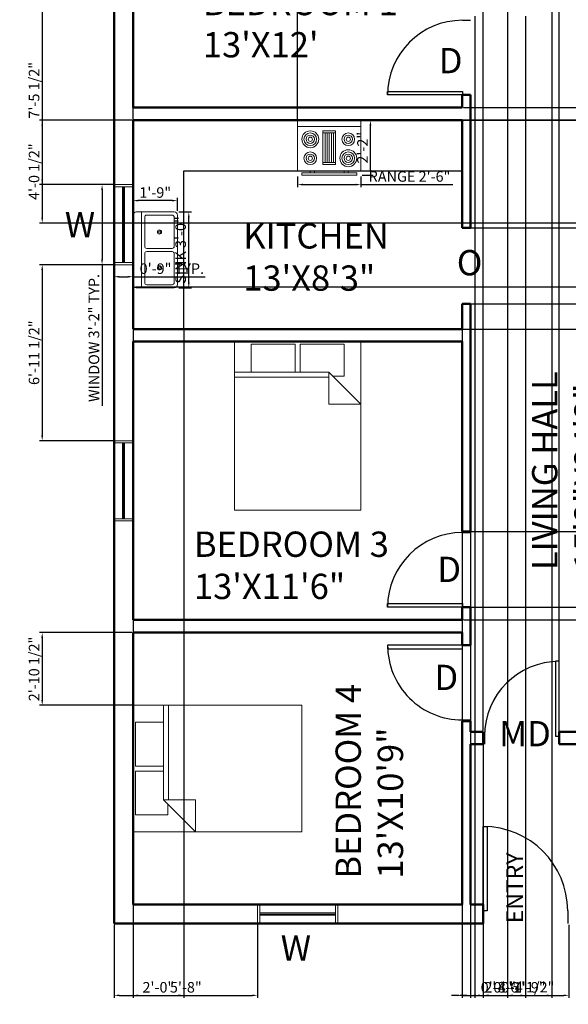
# Model space of a CAD drawing. Units: inches. Extents: x 2050 to 2529, y 1266 to 1968.
# Tile 1 of 5: x 2050 to 2310, y 1266 to 1733. Entities that reach past the tile are written whole.
import ezdxf

# ---------------------------------------------------------------- set-up
doc = ezdxf.new("R2010")
doc.units = ezdxf.units.IN
for name, color, linetype, lineweight in [('A-ANNO-DIMS', 2, 'Continuous', 18), ('A-ANNO-TEXT', 7, 'Continuous', 18), ('A-AREA-IDEN', 7, 'Continuous', 25), ('A-DOOR', 3, 'Continuous', 25), ('A-EQPM', 9, 'Continuous', 18), ('A-FLOR-CABN', 8, 'Continuous', 25), ('A-FLOR-FIXT', 9, 'Continuous', 18), ('A-FURN', 8, 'Continuous', 18), ('A-GLAZ', 4, 'Continuous', 18), ('A-WALL', 7, 'Continuous', 50)]:
    doc.layers.add(name, color=color, linetype=linetype, lineweight=lineweight)
doc.styles.get("Standard").update_dxf_attribs({"font": 'arial.ttf'})
doc.dimstyles.new('ISO-25', dxfattribs={"dimtxt": 5, "dimasz": 2.5, "dimexe": 1.25, "dimexo": 0.625, "dimtad": 1, "dimlunit": 3, "dimtxsty": 'Standard', "dimcen": 2.5, "dimadec": 0, "dimazin": 0, "dimtfac": 1, "dimtmove": 0, "dimatfit": 3, "dimfxl": 1, "dimarcsym": 0})

# ---------------------------------------------------------------- blocks, each defined once
blk = doc.blocks.new('*U4')
for p, q in [((0, 0), (0, -100)), ((-900, 0), (-900, -100))]:
    blk.add_line(p, q)
blk.add_lwpolyline([(0, 0), (0, 900), (-43.75, 900), (-43.75, 0)], close=True)
blk.add_arc((0, 0), 900, 90, 180)
blk = doc.blocks.new('*U5')
for p, q in [((-900, 0), (-900, 100)), ((0, 0), (0, 100))]:
    blk.add_line(p, q)
blk.add_lwpolyline([(0, 0), (0, -900), (-43.75, -900), (-43.75, 0)], close=True)
blk.add_arc((0, 0), 900, 180, 270)
blk = doc.blocks.new('*U6')
for p, q in [((0, 0), (0, 100)), ((900, 0), (900, 100))]:
    blk.add_line(p, q)
blk.add_lwpolyline([(0, 0), (0, -900), (43.75, -900), (43.75, 0)], close=True)
blk.add_arc((0, 0), 900, 270, 0)
blk = doc.blocks.new('*U10')
for p, q in [((0, 0), (0, -6)), ((40, 0), (40, -6))]:
    blk.add_line(p, q)
blk.add_lwpolyline([(0, 0), (0, 40), (1.75, 40), (1.75, 0)], close=True)
blk.add_arc((0, 0), 40, 0, 90)
blk = doc.blocks.new('Sink-double - 36 in top')
for p, q in [((-18, -4), (18, -4)), ((-0.75, -18.5), (-0.75, -6.5)), ((0.75, -6.5), (0.75, -18.5))]:
    blk.add_line(p, q)
for points in [[(-16.5, 0), (16.5, 0)], [(-18, -19.5), (-18, -1.5)], [(18, -1.5), (18, -19.5)], [(-16.5, -18.5), (-16.5, -6.5)], [(-15.5, -5.5), (-1.75, -5.5)], [(1.75, -5.5), (15.5, -5.5)], [(16.5, -6.5), (16.5, -18.5)], [(16.5, -21), (-16.5, -21)], [(-1.75, -19.5), (-15.5, -19.5)], [(15.5, -19.5), (1.75, -19.5)]]:
    blk.add_lwpolyline(points)
for centre, radius in [((-8.5, -12.5), 1), ((-8.5, -12.5), 0.5), ((8.5, -12.5), 1), ((8.5, -12.5), 0.5)]:
    blk.add_circle(centre, radius)
for centre, radius, start, end in [((-16.5, -1.5), 1.5, 90, 180), ((16.5, -1.5), 1.5, 0, 90), ((-15.5, -6.5), 1, 90, 180), ((-1.75, -6.5), 1, 0, 90), ((1.75, -6.5), 1, 90, 180), ((15.5, -6.5), 1, 0, 90), ((-15.5, -18.5), 1, 180, 270), ((-1.75, -18.5), 1, 270, 0), ((1.75, -18.5), 1, 180, 270), ((15.5, -18.5), 1, 270, 0), ((-16.5, -19.5), 1.5, 180, 270), ((16.5, -19.5), 1.5, 270, 0)]:
    blk.add_arc(centre, radius, start, end)
blk = doc.blocks.new('Range-Oven - 30 in top')
for p, q in [((0, -3), (30, -3)), ((12, -6), (18, -6)), ((13, -20), (13, -6)), ((14, -6), (14, -20)), ((15, -20), (15, -6)), ((16, -6), (16, -20)), ((17, -20), (17, -6)), ((18, -20), (12, -20)), ((6, -24), (6, -25)), ((8, -25), (8, -24)), ((22, -25), (22, -24)), ((24, -24), (24, -25))]:
    blk.add_line(p, q)
for points in [[(0, -24), (0, 0), (30, 0), (30, -24)], [(12, -21), (12, -5), (18, -5), (18, -21)], [(2, -26), (2, -25), (28, -25), (28, -26)]]:
    blk.add_lwpolyline(points, close=True)
for centre, radius in [((6, -9), 4), ((6, -9), 3), ((6, -9), 2), ((6, -9), 1), ((24, -9), 3), ((24, -9), 2), ((24, -9), 1), ((24, -18), 4), ((6, -18), 3), ((6, -18), 2), ((6, -18), 1), ((24, -18), 3), ((24, -18), 2), ((24, -18), 1)]:
    blk.add_circle(centre, radius)
blk = doc.blocks.new('Bed - Queen')
for p, q in [((0, -80.00003), (0, 0)), ((0, 0), (59.99999, 0)), ((59.99999, 0), (59.99999, -80.00003)), ((7.99999, -1.2), (28.79998, -1.2)), ((7.99999, -14.4), (7.99999, -1.2)), ((28.79998, -1.2), (28.79998, -14.4)), ((31.19999, -1.2), (51.99999, -1.2)), ((31.19999, -14.4), (31.19999, -1.2)), ((51.99999, -1.2), (51.99999, -16.4)), ((0, -14.4), (44.8, -14.4)), ((44.8, -16.8), (0, -16.8)), ((59.99999, -29.6), (44.8, -14.4)), ((44.8, -14.4), (44.8, -29.6)), ((51.99999, -16.4), (46.79936, -16.4)), ((44.8, -29.6), (59.99999, -29.6)), ((59.99999, -80.00003), (0, -80.00003))]:
    blk.add_line(p, q)
blk = doc.blocks.new('WIN-36IN')
for p, q in [((0, 9), (0, 0)), ((1, 9), (1, 0)), ((1, 5), (37, 5)), ((37, 9), (37, 0)), ((38, 9), (38, 0)), ((1, 4.5), (37, 4.5)), ((1, 4), (37, 4))]:
    blk.add_line(p, q)
blk = doc.blocks.new('*D26')
at = {"layer": 'A-ANNO-DIMS', "color": 0, "lineweight": -2, "transparency": 16777216}
for p, q in [((2093.67, 1655.22), (2087.34, 1655.22)), ((2088.59, 1652.72), (2088.59, 1619.72)), ((2093.67, 1617.22), (2087.34, 1617.22)), ((2088.59, 1617.22), (2088.59, 1550.2))]:
    blk.add_line(p, q, dxfattribs=at)
at = {"layer": 'A-ANNO-DIMS', "color": 0, "transparency": 16777216}
for points in [[(2088.18, 1652.72), (2089.01, 1652.72), (2088.59, 1655.22)], [(2088.18, 1619.72), (2089.01, 1619.72), (2088.59, 1617.22)]]:
    blk.add_solid(points, dxfattribs=at)
at = {"layer": 'Defpoints', "color": 0, "transparency": 16777216}
for p in [(2094.29, 1655.22), (2088.59, 1617.22), (2094.29, 1617.22)]:
    blk.add_point(p, dxfattribs=at)
at = {"layer": 'A-ANNO-DIMS', "color": 0, "transparency": 16777216, "insert": (2085.38, 1582.46), "char_height": 5, "attachment_point": 5, "rotation": 90}
blk.add_mtext('WINDOW 3\'-2" TYP.', dxfattribs=at)
blk = doc.blocks.new('*D27')
at = {"layer": 'A-ANNO-DIMS', "color": 0, "lineweight": -2, "transparency": 16777216}
for p, q in [((2094.29, 1616.6), (2094.29, 1610.27)), ((2103.29, 1616.6), (2103.29, 1610.27)), ((2096.79, 1611.52), (2100.79, 1611.52)), ((2103.29, 1611.52), (2137.52, 1611.52))]:
    blk.add_line(p, q, dxfattribs=at)
at = {"layer": 'A-ANNO-DIMS', "color": 0, "transparency": 16777216}
for points in [[(2096.79, 1611.94), (2096.79, 1611.1), (2094.29, 1611.52)], [(2100.79, 1611.94), (2100.79, 1611.1), (2103.29, 1611.52)]]:
    blk.add_solid(points, dxfattribs=at)
at = {"layer": 'Defpoints', "color": 0, "transparency": 16777216}
for p in [(2094.29, 1617.22), (2103.29, 1617.22), (2103.29, 1611.52)]:
    blk.add_point(p, dxfattribs=at)
at = {"layer": 'A-ANNO-DIMS', "color": 0, "transparency": 16777216, "insert": (2121.66, 1614.7), "char_height": 5, "attachment_point": 5}
blk.add_mtext('0\'-9" TYP.', dxfattribs=at)
blk = doc.blocks.new('*D34')
at = {"layer": 'A-ANNO-DIMS', "color": 0, "lineweight": -2, "transparency": 16777216}
for p, q in [((2124.92, 1642.22), (2130.94, 1642.22)), ((2129.69, 1608.72), (2129.69, 1639.72)), ((2124.92, 1606.22), (2130.94, 1606.22))]:
    blk.add_line(p, q, dxfattribs=at)
at = {"layer": 'A-ANNO-DIMS', "color": 0, "transparency": 16777216}
for points in [[(2129.28, 1639.72), (2130.11, 1639.72), (2129.69, 1642.22)], [(2129.28, 1608.72), (2130.11, 1608.72), (2129.69, 1606.22)]]:
    blk.add_solid(points, dxfattribs=at)
at = {"layer": 'Defpoints', "color": 0, "transparency": 16777216}
for p in [(2124.29, 1642.22), (2129.69, 1642.22), (2124.29, 1606.22)]:
    blk.add_point(p, dxfattribs=at)
at = {"layer": 'A-ANNO-DIMS', "color": 0, "transparency": 16777216, "insert": (2126.48, 1624.22), "char_height": 5, "attachment_point": 5, "rotation": 90}
blk.add_mtext('SINK 3\'-0"', dxfattribs=at)
blk = doc.blocks.new('*D35')
at = {"layer": 'A-ANNO-DIMS', "color": 0, "lineweight": -2, "transparency": 16777216}
for p, q in [((2103.29, 1642.85), (2103.29, 1648.87)), ((2124.29, 1642.85), (2124.29, 1648.87)), ((2121.79, 1647.62), (2105.79, 1647.62))]:
    blk.add_line(p, q, dxfattribs=at)
at = {"layer": 'A-ANNO-DIMS', "color": 0, "transparency": 16777216}
for points in [[(2105.79, 1648.04), (2105.79, 1647.2), (2103.29, 1647.62)], [(2121.79, 1648.04), (2121.79, 1647.2), (2124.29, 1647.62)]]:
    blk.add_solid(points, dxfattribs=at)
at = {"layer": 'Defpoints', "color": 0, "transparency": 16777216}
for p in [(2103.29, 1647.62), (2103.29, 1642.22), (2124.29, 1642.22)]:
    blk.add_point(p, dxfattribs=at)
at = {"layer": 'A-ANNO-DIMS', "color": 0, "transparency": 16777216, "insert": (2113.79, 1650.8), "char_height": 5, "attachment_point": 5}
blk.add_mtext('1\'-9"', dxfattribs=at)
blk = doc.blocks.new('*D36')
at = {"layer": 'A-ANNO-DIMS', "color": 0, "lineweight": -2, "transparency": 16777216}
for p, q in [((2181.29, 1659.1), (2181.29, 1653.97)), ((2211.29, 1659.1), (2211.29, 1653.97)), ((2183.79, 1655.22), (2208.79, 1655.22)), ((2211.29, 1655.22), (2254.86, 1655.22))]:
    blk.add_line(p, q, dxfattribs=at)
at = {"layer": 'A-ANNO-DIMS', "color": 0, "transparency": 16777216}
for points in [[(2183.79, 1655.64), (2183.79, 1654.8), (2181.29, 1655.22)], [(2208.79, 1655.64), (2208.79, 1654.8), (2211.29, 1655.22)]]:
    blk.add_solid(points, dxfattribs=at)
at = {"layer": 'Defpoints', "color": 0, "transparency": 16777216}
for p in [(2181.29, 1659.72), (2211.29, 1659.72), (2211.29, 1655.22)]:
    blk.add_point(p, dxfattribs=at)
at = {"layer": 'A-ANNO-DIMS', "color": 0, "transparency": 16777216, "insert": (2234.33, 1658.43), "char_height": 5, "attachment_point": 5}
blk.add_mtext('RANGE 2\'-6"', dxfattribs=at)
blk = doc.blocks.new('*D37')
at = {"layer": 'A-ANNO-DIMS', "color": 0, "lineweight": -2, "transparency": 16777216}
for p, q in [((2211.92, 1685.72), (2217.04, 1685.72)), ((2215.79, 1662.22), (2215.79, 1683.22)), ((2211.92, 1659.72), (2217.04, 1659.72))]:
    blk.add_line(p, q, dxfattribs=at)
at = {"layer": 'A-ANNO-DIMS', "color": 0, "transparency": 16777216}
for points in [[(2215.38, 1683.22), (2216.21, 1683.22), (2215.79, 1685.72)], [(2215.38, 1662.22), (2216.21, 1662.22), (2215.79, 1659.72)]]:
    blk.add_solid(points, dxfattribs=at)
at = {"layer": 'Defpoints', "color": 0, "transparency": 16777216}
for p in [(2211.29, 1685.72), (2215.79, 1685.72), (2211.29, 1659.72)]:
    blk.add_point(p, dxfattribs=at)
at = {"layer": 'A-ANNO-DIMS', "color": 0, "transparency": 16777216, "insert": (2212.66, 1672.72), "char_height": 5, "attachment_point": 5, "rotation": 90}
blk.add_mtext('2\'-2"', dxfattribs=at)
blk = doc.blocks.new('*D42')
at = {"layer": 'A-ANNO-DIMS', "color": 0, "lineweight": -2, "transparency": 16777216}
for p, q in [((2103.29, 1586.1), (2103.29, 1269.4)), ((2127.29, 1586.1), (2127.29, 1269.4)), ((2105.79, 1270.65), (2124.79, 1270.65))]:
    blk.add_line(p, q, dxfattribs=at)
at = {"layer": 'A-ANNO-DIMS', "color": 0, "transparency": 16777216}
for points in [[(2105.79, 1271.06), (2105.79, 1270.23), (2103.29, 1270.65)], [(2124.79, 1271.06), (2124.79, 1270.23), (2127.29, 1270.65)]]:
    blk.add_solid(points, dxfattribs=at)
at = {"layer": 'Defpoints', "color": 0, "transparency": 16777216}
for p in [(2103.29, 1586.72), (2127.29, 1586.72), (2127.29, 1270.65)]:
    blk.add_point(p, dxfattribs=at)
at = {"layer": 'A-ANNO-DIMS', "color": 0, "transparency": 16777216, "insert": (2115.29, 1273.82), "char_height": 5, "attachment_point": 5}
blk.add_mtext('2\'-0"', dxfattribs=at)
blk = doc.blocks.new('*D43')
at = {"layer": 'A-ANNO-DIMS', "color": 0, "lineweight": -2, "transparency": 16777216}
for p, q in [((2103.29, 1686.35), (2103.29, 1907.05)), ((2105.79, 1905.8), (2178.79, 1905.8)), ((2181.29, 1686.35), (2181.29, 1907.05))]:
    blk.add_line(p, q, dxfattribs=at)
at = {"layer": 'A-ANNO-DIMS', "color": 0, "transparency": 16777216}
for points in [[(2105.79, 1906.21), (2105.79, 1905.38), (2103.29, 1905.8)], [(2178.79, 1906.21), (2178.79, 1905.38), (2181.29, 1905.8)]]:
    blk.add_solid(points, dxfattribs=at)
at = {"layer": 'Defpoints', "color": 0, "transparency": 16777216}
for p in [(2181.29, 1905.8), (2103.29, 1685.72), (2181.29, 1685.72)]:
    blk.add_point(p, dxfattribs=at)
at = {"layer": 'A-ANNO-DIMS', "color": 0, "transparency": 16777216, "insert": (2142.29, 1908.97), "char_height": 5, "attachment_point": 5}
blk.add_mtext('6\'-6"', dxfattribs=at)
blk = doc.blocks.new('*D44')
at = {"layer": 'A-ANNO-DIMS', "color": 0, "lineweight": -2, "transparency": 16777216}
for p, q in [((2104.36, 1606.66), (2489.62, 1606.66)), ((2488.37, 1589.22), (2488.37, 1604.16)), ((2103.92, 1586.72), (2489.62, 1586.72))]:
    blk.add_line(p, q, dxfattribs=at)
at = {"layer": 'A-ANNO-DIMS', "color": 0, "transparency": 16777216}
for points in [[(2487.95, 1604.16), (2488.79, 1604.16), (2488.37, 1606.66)], [(2487.95, 1589.22), (2488.79, 1589.22), (2488.37, 1586.72)]]:
    blk.add_solid(points, dxfattribs=at)
at = {"layer": 'Defpoints', "color": 0, "transparency": 16777216}
for p in [(2103.73, 1606.66), (2488.37, 1606.66), (2103.29, 1586.72)]:
    blk.add_point(p, dxfattribs=at)
at = {"layer": 'A-ANNO-DIMS', "color": 0, "transparency": 16777216, "insert": (2485.19, 1596.69), "char_height": 5, "attachment_point": 5, "rotation": 90}
blk.add_mtext('1\'-8"', dxfattribs=at)
blk = doc.blocks.new('*D45')
at = {"layer": 'A-ANNO-DIMS', "color": 0, "lineweight": -2, "transparency": 16777216}
for p, q in [((2259.92, 1634.72), (2489.62, 1634.72)), ((2488.37, 1601.22), (2488.37, 1632.22)), ((2259.92, 1598.72), (2489.62, 1598.72))]:
    blk.add_line(p, q, dxfattribs=at)
at = {"layer": 'A-ANNO-DIMS', "color": 0, "transparency": 16777216}
for points in [[(2487.95, 1632.22), (2488.79, 1632.22), (2488.37, 1634.72)], [(2487.95, 1601.22), (2488.79, 1601.22), (2488.37, 1598.72)]]:
    blk.add_solid(points, dxfattribs=at)
at = {"layer": 'Defpoints', "color": 0, "transparency": 16777216}
for p in [(2259.29, 1634.72), (2488.37, 1634.72), (2259.29, 1598.72)]:
    blk.add_point(p, dxfattribs=at)
at = {"layer": 'A-ANNO-DIMS', "color": 0, "transparency": 16777216, "insert": (2485.19, 1616.72), "char_height": 5, "attachment_point": 5, "rotation": 90}
blk.add_mtext('3\'-0"', dxfattribs=at)
blk = doc.blocks.new('*D46')
at = {"layer": 'A-ANNO-DIMS', "color": 0, "lineweight": -2, "transparency": 16777216}
for p, q in [((2259.29, 1598.1), (2259.29, 1269.4)), ((2263.29, 1598.1), (2263.29, 1269.4)), ((2256.79, 1270.65), (2254.29, 1270.65)), ((2259.29, 1270.65), (2263.29, 1270.65)), ((2265.79, 1270.65), (2282.84, 1270.65))]:
    blk.add_line(p, q, dxfattribs=at)
at = {"layer": 'A-ANNO-DIMS', "color": 0, "transparency": 16777216}
for points in [[(2256.79, 1271.06), (2256.79, 1270.23), (2259.29, 1270.65)], [(2265.79, 1271.06), (2265.79, 1270.23), (2263.29, 1270.65)]]:
    blk.add_solid(points, dxfattribs=at)
at = {"layer": 'Defpoints', "color": 0, "transparency": 16777216}
for p in [(2259.29, 1598.72), (2263.29, 1598.72), (2263.29, 1270.65)]:
    blk.add_point(p, dxfattribs=at)
at = {"layer": 'A-ANNO-DIMS', "color": 0, "transparency": 16777216, "insert": (2275.57, 1273.82), "char_height": 5, "attachment_point": 5}
blk.add_mtext('0\'-4"', dxfattribs=at)
blk = doc.blocks.new('*D47')
at = {"layer": 'A-ANNO-DIMS', "color": 0, "lineweight": -2, "transparency": 16777216}
for p, q in [((2488.37, 1598.72), (2488.37, 1615.29)), ((2259.92, 1598.72), (2489.62, 1598.72)), ((2488.37, 1589.22), (2488.37, 1596.22)), ((2259.92, 1586.72), (2489.62, 1586.72))]:
    blk.add_line(p, q, dxfattribs=at)
at = {"layer": 'A-ANNO-DIMS', "color": 0, "transparency": 16777216}
for points in [[(2487.95, 1596.22), (2488.79, 1596.22), (2488.37, 1598.72)], [(2487.95, 1589.22), (2488.79, 1589.22), (2488.37, 1586.72)]]:
    blk.add_solid(points, dxfattribs=at)
at = {"layer": 'Defpoints', "color": 0, "transparency": 16777216}
for p in [(2259.29, 1598.72), (2488.37, 1598.72), (2259.29, 1586.72)]:
    blk.add_point(p, dxfattribs=at)
at = {"layer": 'A-ANNO-DIMS', "color": 0, "transparency": 16777216, "insert": (2485.19, 1608.26), "char_height": 5, "attachment_point": 5, "rotation": 90}
blk.add_mtext('1\'-0"', dxfattribs=at)
blk = doc.blocks.new('*D48')
at = {"layer": 'A-ANNO-DIMS', "color": 0, "lineweight": -2, "transparency": 16777216}
for p, q in [((2488.37, 1694.22), (2488.37, 1711.26)), ((2259.92, 1691.72), (2489.62, 1691.72)), ((2488.37, 1685.72), (2488.37, 1691.72)), ((2259.92, 1685.72), (2489.62, 1685.72)), ((2488.37, 1683.22), (2488.37, 1680.72))]:
    blk.add_line(p, q, dxfattribs=at)
at = {"layer": 'A-ANNO-DIMS', "color": 0, "transparency": 16777216}
for points in [[(2487.95, 1694.22), (2488.79, 1694.22), (2488.37, 1691.72)], [(2487.95, 1683.22), (2488.79, 1683.22), (2488.37, 1685.72)]]:
    blk.add_solid(points, dxfattribs=at)
at = {"layer": 'Defpoints', "color": 0, "transparency": 16777216}
for p in [(2259.29, 1691.72), (2488.37, 1691.72), (2259.29, 1685.72)]:
    blk.add_point(p, dxfattribs=at)
at = {"layer": 'A-ANNO-DIMS', "color": 0, "transparency": 16777216, "insert": (2485.19, 1703.99), "char_height": 5, "attachment_point": 5, "rotation": 90}
blk.add_mtext('0\'-6"', dxfattribs=at)
blk = doc.blocks.new('*D49')
at = {"layer": 'A-ANNO-DIMS', "color": 0, "lineweight": -2, "transparency": 16777216}
for p, q in [((2269.29, 1304.1), (2269.29, 1269.4)), ((2309.85, 1304.1), (2309.85, 1269.4)), ((2271.79, 1270.65), (2307.35, 1270.65))]:
    blk.add_line(p, q, dxfattribs=at)
at = {"layer": 'A-ANNO-DIMS', "color": 0, "transparency": 16777216}
for points in [[(2271.79, 1271.06), (2271.79, 1270.23), (2269.29, 1270.65)], [(2307.35, 1271.06), (2307.35, 1270.23), (2309.85, 1270.65)]]:
    blk.add_solid(points, dxfattribs=at)
at = {"layer": 'Defpoints', "color": 0, "transparency": 16777216}
for p in [(2269.29, 1304.72), (2309.85, 1304.72), (2309.85, 1270.65)]:
    blk.add_point(p, dxfattribs=at)
at = {"layer": 'A-ANNO-DIMS', "color": 0, "transparency": 16777216, "insert": (2289.57, 1273.86), "char_height": 5, "attachment_point": 5}
blk.add_mtext('3\'-4 1/2"', dxfattribs=at)
blk = doc.blocks.new('*D50')
at = {"layer": 'A-ANNO-DIMS', "color": 0, "lineweight": -2, "transparency": 16777216}
for p, q in [((2263.29, 1313.1), (2263.29, 1269.4)), ((2269.29, 1313.1), (2269.29, 1269.4)), ((2260.79, 1270.65), (2258.29, 1270.65)), ((2263.29, 1270.65), (2269.29, 1270.65)), ((2271.79, 1270.65), (2288.84, 1270.65))]:
    blk.add_line(p, q, dxfattribs=at)
at = {"layer": 'A-ANNO-DIMS', "color": 0, "transparency": 16777216}
for points in [[(2260.79, 1271.06), (2260.79, 1270.23), (2263.29, 1270.65)], [(2271.79, 1271.06), (2271.79, 1270.23), (2269.29, 1270.65)]]:
    blk.add_solid(points, dxfattribs=at)
at = {"layer": 'Defpoints', "color": 0, "transparency": 16777216}
for p in [(2263.29, 1313.72), (2269.29, 1313.72), (2269.29, 1270.65)]:
    blk.add_point(p, dxfattribs=at)
at = {"layer": 'A-ANNO-DIMS', "color": 0, "transparency": 16777216, "insert": (2281.57, 1273.82), "char_height": 5, "attachment_point": 5}
blk.add_mtext('0\'-6"', dxfattribs=at)
blk = doc.blocks.new('*D54')
at = {"layer": 'A-ANNO-DIMS', "color": 0, "lineweight": -2, "transparency": 16777216}
for p, q in [((2269.29, 1396.35), (2269.29, 1907.05)), ((2271.79, 1905.8), (2302.79, 1905.8)), ((2305.29, 1396.35), (2305.29, 1907.05))]:
    blk.add_line(p, q, dxfattribs=at)
at = {"layer": 'A-ANNO-DIMS', "color": 0, "transparency": 16777216}
for points in [[(2271.79, 1906.21), (2271.79, 1905.38), (2269.29, 1905.8)], [(2302.79, 1906.21), (2302.79, 1905.38), (2305.29, 1905.8)]]:
    blk.add_solid(points, dxfattribs=at)
at = {"layer": 'Defpoints', "color": 0, "transparency": 16777216}
for p in [(2305.29, 1905.8), (2269.29, 1395.72), (2305.29, 1395.72)]:
    blk.add_point(p, dxfattribs=at)
at = {"layer": 'A-ANNO-DIMS', "color": 0, "transparency": 16777216, "insert": (2287.29, 1908.98), "char_height": 5, "attachment_point": 5}
blk.add_mtext('3\'-0"', dxfattribs=at)
blk = doc.blocks.new('*D55')
at = {"layer": 'A-ANNO-DIMS', "color": 0, "lineweight": -2, "transparency": 16777216}
for p, q in [((2263.29, 1395.1), (2263.29, 1269.4)), ((2269.29, 1395.1), (2269.29, 1269.4)), ((2260.79, 1270.65), (2258.29, 1270.65)), ((2263.29, 1270.65), (2269.29, 1270.65)), ((2271.79, 1270.65), (2288.84, 1270.65))]:
    blk.add_line(p, q, dxfattribs=at)
at = {"layer": 'A-ANNO-DIMS', "color": 0, "transparency": 16777216}
for points in [[(2260.79, 1271.06), (2260.79, 1270.23), (2263.29, 1270.65)], [(2271.79, 1271.06), (2271.79, 1270.23), (2269.29, 1270.65)]]:
    blk.add_solid(points, dxfattribs=at)
at = {"layer": 'Defpoints', "color": 0, "transparency": 16777216}
for p in [(2263.29, 1395.72), (2269.29, 1395.72), (2269.29, 1270.65)]:
    blk.add_point(p, dxfattribs=at)
at = {"layer": 'A-ANNO-DIMS', "color": 0, "transparency": 16777216, "insert": (2281.57, 1273.82), "char_height": 5, "attachment_point": 5}
blk.add_mtext('0\'-6"', dxfattribs=at)
blk = doc.blocks.new('*D58')
at = {"layer": 'A-ANNO-DIMS', "color": 0, "lineweight": -2, "transparency": 16777216}
for p, q in [((2488.37, 1457.22), (2488.37, 1474.26)), ((2259.92, 1454.72), (2489.62, 1454.72)), ((2488.37, 1448.72), (2488.37, 1454.72)), ((2259.92, 1448.72), (2489.62, 1448.72)), ((2488.37, 1446.22), (2488.37, 1443.72))]:
    blk.add_line(p, q, dxfattribs=at)
at = {"layer": 'A-ANNO-DIMS', "color": 0, "transparency": 16777216}
for points in [[(2487.95, 1457.22), (2488.79, 1457.22), (2488.37, 1454.72)], [(2487.95, 1446.22), (2488.79, 1446.22), (2488.37, 1448.72)]]:
    blk.add_solid(points, dxfattribs=at)
at = {"layer": 'Defpoints', "color": 0, "transparency": 16777216}
for p in [(2259.29, 1454.72), (2488.37, 1454.72), (2259.29, 1448.72)]:
    blk.add_point(p, dxfattribs=at)
at = {"layer": 'A-ANNO-DIMS', "color": 0, "transparency": 16777216, "insert": (2485.19, 1466.99), "char_height": 5, "attachment_point": 5, "rotation": 90}
blk.add_mtext('0\'-6"', dxfattribs=at)
blk = doc.blocks.new('*D59')
at = {"layer": 'A-ANNO-DIMS', "color": 0, "lineweight": -2, "transparency": 16777216}
for p, q in [((2259.92, 1490.72), (2489.62, 1490.72)), ((2488.37, 1457.22), (2488.37, 1488.22)), ((2259.92, 1454.72), (2489.62, 1454.72))]:
    blk.add_line(p, q, dxfattribs=at)
at = {"layer": 'A-ANNO-DIMS', "color": 0, "transparency": 16777216}
for points in [[(2487.95, 1488.22), (2488.79, 1488.22), (2488.37, 1490.72)], [(2487.95, 1457.22), (2488.79, 1457.22), (2488.37, 1454.72)]]:
    blk.add_solid(points, dxfattribs=at)
at = {"layer": 'Defpoints', "color": 0, "transparency": 16777216}
for p in [(2259.29, 1490.72), (2488.37, 1490.72), (2259.29, 1454.72)]:
    blk.add_point(p, dxfattribs=at)
at = {"layer": 'A-ANNO-DIMS', "color": 0, "transparency": 16777216, "insert": (2485.19, 1472.72), "char_height": 5, "attachment_point": 5, "rotation": 90}
blk.add_mtext('3\'-0"', dxfattribs=at)
blk = doc.blocks.new('*D60')
at = {"layer": 'A-ANNO-DIMS', "color": 0, "lineweight": -2, "transparency": 16777216}
for p, q in [((2265.29, 1735.1), (2265.29, 1269.4)), ((2289.29, 1735.1), (2289.29, 1269.4)), ((2267.79, 1270.65), (2286.79, 1270.65))]:
    blk.add_line(p, q, dxfattribs=at)
at = {"layer": 'A-ANNO-DIMS', "color": 0, "transparency": 16777216}
for points in [[(2267.79, 1271.06), (2267.79, 1270.23), (2265.29, 1270.65)], [(2286.79, 1271.06), (2286.79, 1270.23), (2289.29, 1270.65)]]:
    blk.add_solid(points, dxfattribs=at)
at = {"layer": 'Defpoints', "color": 0, "transparency": 16777216}
for p in [(2265.29, 1735.72), (2289.29, 1735.72), (2289.29, 1270.65)]:
    blk.add_point(p, dxfattribs=at)
at = {"layer": 'A-ANNO-DIMS', "color": 0, "transparency": 16777216, "insert": (2277.29, 1273.82), "char_height": 5, "attachment_point": 5}
blk.add_mtext('2\'-0"', dxfattribs=at)
blk = doc.blocks.new('*D64')
at = {"layer": 'A-ANNO-DIMS', "color": 0, "lineweight": -2, "transparency": 16777216}
for p, q in [((2280.79, 1835.1), (2280.79, 1269.4)), ((2301.79, 1835.1), (2301.79, 1269.4)), ((2283.29, 1270.65), (2299.29, 1270.65))]:
    blk.add_line(p, q, dxfattribs=at)
at = {"layer": 'A-ANNO-DIMS', "color": 0, "transparency": 16777216}
for points in [[(2283.29, 1271.06), (2283.29, 1270.23), (2280.79, 1270.65)], [(2299.29, 1271.06), (2299.29, 1270.23), (2301.79, 1270.65)]]:
    blk.add_solid(points, dxfattribs=at)
at = {"layer": 'Defpoints', "color": 0, "transparency": 16777216}
for p in [(2280.79, 1835.72), (2301.79, 1835.72), (2301.79, 1270.65)]:
    blk.add_point(p, dxfattribs=at)
at = {"layer": 'A-ANNO-DIMS', "color": 0, "transparency": 16777216, "insert": (2291.29, 1273.82), "char_height": 5, "attachment_point": 5}
blk.add_mtext('1\'-9"', dxfattribs=at)
blk = doc.blocks.new('*D67')
at = {"layer": 'A-ANNO-DIMS', "color": 0, "lineweight": -2, "transparency": 16777216}
for p, q in [((2093.67, 1744.72), (2058.97, 1744.72)), ((2060.22, 1742.22), (2060.22, 1657.72)), ((2093.67, 1655.22), (2058.97, 1655.22))]:
    blk.add_line(p, q, dxfattribs=at)
at = {"layer": 'A-ANNO-DIMS', "color": 0, "transparency": 16777216}
for points in [[(2059.8, 1742.22), (2060.64, 1742.22), (2060.22, 1744.72)], [(2059.8, 1657.72), (2060.64, 1657.72), (2060.22, 1655.22)]]:
    blk.add_solid(points, dxfattribs=at)
at = {"layer": 'Defpoints', "color": 0, "transparency": 16777216}
for p in [(2094.29, 1744.72), (2060.22, 1655.22), (2094.29, 1655.22)]:
    blk.add_point(p, dxfattribs=at)
at = {"layer": 'A-ANNO-DIMS', "color": 0, "transparency": 16777216, "insert": (2057.01, 1699.97), "char_height": 5, "attachment_point": 5, "rotation": 90}
blk.add_mtext('7\'-5 1/2"', dxfattribs=at)
blk = doc.blocks.new('*D68')
at = {"layer": 'A-ANNO-DIMS', "color": 0, "lineweight": -2, "transparency": 16777216}
for p, q in [((2093.67, 1617.22), (2058.97, 1617.22)), ((2060.22, 1614.72), (2060.22, 1536.22)), ((2093.67, 1533.72), (2058.97, 1533.72))]:
    blk.add_line(p, q, dxfattribs=at)
at = {"layer": 'A-ANNO-DIMS', "color": 0, "transparency": 16777216}
for points in [[(2059.8, 1614.72), (2060.64, 1614.72), (2060.22, 1617.22)], [(2059.8, 1536.22), (2060.64, 1536.22), (2060.22, 1533.72)]]:
    blk.add_solid(points, dxfattribs=at)
at = {"layer": 'Defpoints', "color": 0, "transparency": 16777216}
for p in [(2094.29, 1617.22), (2060.22, 1533.72), (2094.29, 1533.72)]:
    blk.add_point(p, dxfattribs=at)
at = {"layer": 'A-ANNO-DIMS', "color": 0, "transparency": 16777216, "insert": (2057.01, 1575.47), "char_height": 5, "attachment_point": 5, "rotation": 90}
blk.add_mtext('6\'-11 1/2"', dxfattribs=at)
blk = doc.blocks.new('*D69')
at = {"layer": 'A-ANNO-DIMS', "color": 0, "lineweight": -2, "transparency": 16777216}
for p, q in [((2094.29, 1304.1), (2094.29, 1269.4)), ((2162.29, 1304.1), (2162.29, 1269.4)), ((2096.79, 1270.65), (2159.79, 1270.65))]:
    blk.add_line(p, q, dxfattribs=at)
at = {"layer": 'A-ANNO-DIMS', "color": 0, "transparency": 16777216}
for points in [[(2096.79, 1271.06), (2096.79, 1270.23), (2094.29, 1270.65)], [(2159.79, 1271.06), (2159.79, 1270.23), (2162.29, 1270.65)]]:
    blk.add_solid(points, dxfattribs=at)
at = {"layer": 'Defpoints', "color": 0, "transparency": 16777216}
for p in [(2094.29, 1304.72), (2162.29, 1304.72), (2162.29, 1270.65)]:
    blk.add_point(p, dxfattribs=at)
at = {"layer": 'A-ANNO-DIMS', "color": 0, "transparency": 16777216, "insert": (2128.29, 1273.82), "char_height": 5, "attachment_point": 5}
blk.add_mtext('5\'-8"', dxfattribs=at)
blk = doc.blocks.new('*D76')
at = {"layer": 'A-ANNO-DIMS', "color": 0, "lineweight": -2, "transparency": 16777216}
for p, q in [((2102.67, 1442.72), (2058.97, 1442.72)), ((2060.22, 1440.22), (2060.22, 1410.72)), ((2102.67, 1408.22), (2058.97, 1408.22))]:
    blk.add_line(p, q, dxfattribs=at)
at = {"layer": 'A-ANNO-DIMS', "color": 0, "transparency": 16777216}
for points in [[(2059.8, 1440.22), (2060.64, 1440.22), (2060.22, 1442.72)], [(2059.8, 1410.72), (2060.64, 1410.72), (2060.22, 1408.22)]]:
    blk.add_solid(points, dxfattribs=at)
at = {"layer": 'Defpoints', "color": 0, "transparency": 16777216}
for p in [(2103.29, 1442.72), (2060.22, 1408.22), (2103.29, 1408.22)]:
    blk.add_point(p, dxfattribs=at)
at = {"layer": 'A-ANNO-DIMS', "color": 0, "transparency": 16777216, "insert": (2057.01, 1425.47), "char_height": 5, "attachment_point": 5, "rotation": 90}
blk.add_mtext('2\'-10 1/2"', dxfattribs=at)
blk = doc.blocks.new('*D78')
at = {"layer": 'A-ANNO-DIMS', "color": 0, "lineweight": -2, "transparency": 16777216}
for p, q in [((2318.67, 1685.72), (2058.97, 1685.72)), ((2060.22, 1683.22), (2060.22, 1639.48)), ((2329.62, 1636.98), (2058.97, 1636.98))]:
    blk.add_line(p, q, dxfattribs=at)
at = {"layer": 'A-ANNO-DIMS', "color": 0, "transparency": 16777216}
for points in [[(2059.8, 1683.22), (2060.64, 1683.22), (2060.22, 1685.72)], [(2059.8, 1639.48), (2060.64, 1639.48), (2060.22, 1636.98)]]:
    blk.add_solid(points, dxfattribs=at)
at = {"layer": 'Defpoints', "color": 0, "transparency": 16777216}
for p in [(2319.29, 1685.72), (2060.22, 1636.98), (2330.24, 1636.98)]:
    blk.add_point(p, dxfattribs=at)
at = {"layer": 'A-ANNO-DIMS', "color": 0, "transparency": 16777216, "insert": (2057.01, 1661.35), "char_height": 5, "attachment_point": 5, "rotation": 90}
blk.add_mtext('4\'-0 1/2"', dxfattribs=at)

msp = doc.modelspace()

# ---------------------------------------------------------------- linework, layer by layer
at = {"layer": 'A-FLOR-CABN'}
for p, q in [((2127.295, 1586.72), (2127.295, 1661.72)), ((2127.295, 1661.72), (2259.295, 1661.72))]:
    msp.add_line(p, q, dxfattribs=at)
at = {"layer": 'A-WALL'}
for p, q in [((2094.295, 1304.72), (2094.295, 1844.72)), ((2103.295, 1691.72), (2103.295, 1835.72)), ((2259.295, 1697.72), (2263.295, 1697.72)), ((2259.295, 1691.72), (2259.295, 1697.72)), ((2263.295, 1634.72), (2263.295, 1697.72)), ((2103.295, 1691.72), (2259.295, 1691.72)), ((2103.295, 1685.72), (2259.295, 1685.72)), ((2103.295, 1586.72), (2103.295, 1685.72)), ((2259.295, 1634.72), (2259.295, 1685.72)), ((2259.295, 1634.72), (2263.295, 1634.72)), ((2259.295, 1598.72), (2263.295, 1598.72)), ((2259.295, 1586.72), (2259.295, 1598.72)), ((2263.295, 1490.72), (2263.295, 1598.72)), ((2103.295, 1586.72), (2259.295, 1586.72)), ((2103.295, 1580.72), (2259.295, 1580.72)), ((2103.295, 1448.72), (2103.295, 1580.72)), ((2259.295, 1490.72), (2259.295, 1580.72)), ((2259.295, 1490.72), (2263.295, 1490.72)), ((2259.295, 1454.72), (2263.295, 1454.72)), ((2259.295, 1448.72), (2259.295, 1454.72)), ((2263.295, 1436.72), (2263.295, 1454.72)), ((2103.295, 1448.72), (2259.295, 1448.72)), ((2103.295, 1313.72), (2103.295, 1442.72)), ((2103.295, 1442.72), (2259.295, 1442.72)), ((2103.295, 1442.72), (2103.295, 1313.72)), ((2259.295, 1436.72), (2259.295, 1442.72)), ((2259.295, 1436.72), (2263.295, 1436.72)), ((2259.295, 1313.72), (2259.295, 1400.72)), ((2259.295, 1400.72), (2263.295, 1400.72)), ((2263.295, 1395.72), (2263.295, 1400.72)), ((2263.295, 1395.72), (2269.295, 1395.72)), ((2269.295, 1395.72), (2269.295, 1389.72)), ((2305.295, 1395.72), (2305.295, 1389.72)), ((2305.295, 1395.72), (2445.295, 1395.72)), ((2263.295, 1313.72), (2263.295, 1389.72)), ((2263.295, 1389.72), (2269.295, 1389.72)), ((2305.295, 1389.72), (2445.295, 1389.72)), ((2259.295, 1313.72), (2103.295, 1313.72)), ((2269.295, 1313.72), (2263.295, 1313.72)), ((2269.295, 1313.72), (2269.295, 1304.72)), ((2269.295, 1304.72), (2094.295, 1304.72))]:
    msp.add_line(p, q, dxfattribs=at)

# ---------------------------------------------------------------- block references
at = {"layer": 'A-DOOR', "xscale": 0.0393700787401575, "yscale": 0.0393700787401575, "zscale": 0.0393700787401575, "rotation": 270}
for name, p in [('*U5', (2259.358, 1697.72)), ('*U5', (2259.358, 1454.72)), ('*U6', (2259.358, 1436.72))]:
    msp.add_blockref(name, p, dxfattribs=at)
at = {"layer": 'A-DOOR', "xscale": 0.0393700787401575, "yscale": 0.0393700787401575, "zscale": 0.0393700787401575}
msp.add_blockref('*U4', (2305.295, 1393.657), dxfattribs=at)
at = {"layer": 'A-DOOR'}
msp.add_blockref('*U10', (2269.295, 1310.72), dxfattribs=at)
at = {"layer": 'A-EQPM'}
msp.add_blockref('Range-Oven - 30 in top', (2181.295, 1685.72), dxfattribs=at)
at = {"layer": 'A-FLOR-FIXT', "rotation": 90}
msp.add_blockref('Sink-double - 36 in top', (2103.295, 1624.22), dxfattribs=at)
at = {"layer": 'A-FURN'}
msp.add_blockref('Bed - Queen', (2151.295, 1580.72), dxfattribs=at)
at = {"layer": 'A-FURN', "xscale": -1, "rotation": 90}
msp.add_blockref('Bed - Queen', (2103.295, 1408.22), dxfattribs=at)
at = {"layer": 'A-GLAZ', "rotation": 269.9999999999973}
for p in [(2094.294, 1655.22), (2094.294, 1533.72)]:
    msp.add_blockref('WIN-36IN', p, dxfattribs=at)
at = {"layer": 'A-GLAZ'}
msp.add_blockref('WIN-36IN', (2162.295, 1304.72), dxfattribs=at)

# ---------------------------------------------------------------- texts
at = {"layer": 'A-ANNO-TEXT', "char_height": 12, "attachment_point": 1}
for s, insert in [('D', (2248.179, 1720.023)), ('W', (2070.929, 1642.261)), ('O', (2256.716, 1624.175)), ('D', (2247.472, 1478.695)), ('D', (2246.104, 1427.449)), ('MD', (2276.755, 1400.773)), ('W', (2173.261, 1299.102))]:
    msp.add_mtext_dynamic_manual_height_columns(s, width=471.52273, gutter_width=12.5, heights=[28.462], dxfattribs=dict(at, insert=insert))
at = {"layer": 'A-AREA-IDEN', "char_height": 12, "attachment_point": 1}
for s, insert in [("BEDROOM 1\\P13'X12'", (2136.374, 1747.567)), ('KITCHEN\\P13\'X8\'3"', (2155.508, 1636.878)), ('BEDROOM 3\\P13\'X11\'6"', (2132.149, 1490.638))]:
    msp.add_mtext_dynamic_manual_height_columns(s, width=649.2389, gutter_width=12.5, heights=[75.088], dxfattribs=dict(at, insert=insert))
at = {"layer": 'A-AREA-IDEN', "attachment_point": 1, "rotation": 90}
for s, insert, char_height in [('LIVING HALL\\P15\'2"X24\'2"', (2292.409, 1472.375), 12), ('BEDROOM 4\\P13\'X10\'9"', (2199.261, 1326.016), 12), ('ENTRY', (2280.172, 1304.841), 8)]:
    msp.add_mtext_dynamic_manual_height_columns(s, width=649.2389, gutter_width=12.5, heights=[75.088], dxfattribs=dict(at, insert=insert, char_height=char_height))

# ---------------------------------------------------------------- dimensions: what is measured, and where the dimension line sits
at = {"layer": 'A-ANNO-DIMS'}
for base, p1, p2, picture, middle in [((2181.295, 1905.795), (2103.295, 1685.72), (2181.295, 1685.72), '*D43', (2142.295, 1908.973)), ((2305.295, 1905.795), (2269.295, 1395.72), (2305.295, 1395.72), '*D54', (2287.295, 1908.975)), ((2301.795, 1270.645), (2280.795, 1835.72), (2301.795, 1835.72), '*D64', (2291.295, 1273.823)), ((2289.295, 1270.645), (2265.295, 1735.72), (2289.295, 1735.72), '*D60', (2277.295, 1273.823)), ((2263.295, 1270.645), (2259.295, 1598.72), (2263.295, 1598.72), '*D46', (2275.565, 1273.823)), ((2127.295, 1270.645), (2103.295, 1586.72), (2127.295, 1586.72), '*D42', (2115.295, 1273.823)), ((2269.295, 1270.645), (2263.295, 1395.72), (2269.295, 1395.72), '*D55', (2281.565, 1273.823)), ((2269.295, 1270.645), (2263.295, 1313.72), (2269.295, 1313.72), '*D50', (2281.565, 1273.823)), ((2162.295, 1270.645), (2094.295, 1304.72), (2162.295, 1304.72), '*D69', (2128.295, 1273.823)), ((2309.846, 1270.645), (2269.295, 1304.72), (2309.846, 1304.72), '*D49', (2289.57, 1273.857))]:
    dim = msp.add_linear_dim(base=base, p1=p1, p2=p2, dimstyle='ISO-25', override={"dimdec": 1, "dimlfac": 1, "dimrnd": 0, "dimzin": 1, "dimdsep": 46, "dimlunit": 4, "dimfrac": 2}, dxfattribs=at)
    dim.commit()
    dim.dimension.update_dxf_attribs({"geometry": picture, "text_midpoint": middle})
for base, p1, p2, angle, picture, middle in [((2060.22, 1655.22), (2094.295, 1744.72), (2094.295, 1655.22), 90, '*D67', (2057.009, 1699.97)), ((2488.37, 1691.72), (2259.295, 1685.72), (2259.295, 1691.72), 90, '*D48', (2485.192, 1703.991)), ((2060.22, 1636.982), (2319.295, 1685.72), (2330.24, 1636.982), 90, '*D78', (2057.009, 1661.351)), ((2215.795, 1685.72), (2211.295, 1659.72), (2211.295, 1685.72), 90, '*D37', (2212.659, 1672.72)), ((2103.295, 1647.62), (2124.295, 1642.22), (2103.295, 1642.22), 180, '*D35', (2113.795, 1650.798)), ((2488.37, 1634.72), (2259.295, 1598.72), (2259.295, 1634.72), 90, '*D45', (2485.19, 1616.72)), ((2060.22, 1533.72), (2094.295, 1617.22), (2094.295, 1533.72), 90, '*D68', (2057.009, 1575.47)), ((2488.37, 1598.72), (2259.295, 1586.72), (2259.295, 1598.72), 90, '*D47', (2485.192, 1608.256)), ((2488.37, 1606.66), (2103.295, 1586.72), (2103.734, 1606.66), 90, '*D44', (2485.192, 1596.69)), ((2488.37, 1490.72), (2259.295, 1454.72), (2259.295, 1490.72), 90, '*D59', (2485.19, 1472.72)), ((2488.37, 1454.72), (2259.295, 1448.72), (2259.295, 1454.72), 90, '*D58', (2485.192, 1466.991)), ((2060.22, 1408.22), (2103.295, 1442.72), (2103.295, 1408.22), 90, '*D76', (2057.009, 1425.47))]:
    dim = msp.add_linear_dim(base=base, p1=p1, p2=p2, angle=angle, dimstyle='ISO-25', override={"dimdec": 1, "dimlfac": 1, "dimrnd": 0, "dimzin": 1, "dimdsep": 46, "dimlunit": 4, "dimfrac": 2}, dxfattribs=at)
    dim.commit()
    dim.dimension.update_dxf_attribs({"geometry": picture, "text_midpoint": middle})
for base, p1, p2, text, picture, middle in [((2211.295, 1655.22), (2181.295, 1659.72), (2211.295, 1659.72), 'RANGE <>', '*D36', (2234.326, 1658.431)), ((2103.295, 1611.52), (2094.295, 1617.22), (2103.295, 1617.22), '<> TYP.', '*D27', (2121.658, 1614.698))]:
    dim = msp.add_linear_dim(base=base, p1=p1, p2=p2, text=text, dimstyle='ISO-25', override={"dimdec": 1, "dimlfac": 1, "dimrnd": 0, "dimzin": 1, "dimdsep": 46, "dimlunit": 4, "dimfrac": 2}, dxfattribs=at)
    dim.commit()
    dim.dimension.update_dxf_attribs({"geometry": picture, "text_midpoint": middle})
for base, p1, p2, angle, text, picture, middle in [((2088.595, 1617.22), (2094.295, 1655.22), (2094.295, 1617.22), 270, 'WINDOW <> TYP.', '*D26', (2085.381, 1582.46)), ((2129.695, 1642.22), (2124.295, 1606.22), (2124.295, 1642.22), 90, 'SINK <>', '*D34', (2126.483, 1624.22))]:
    dim = msp.add_linear_dim(base=base, p1=p1, p2=p2, angle=angle, text=text, dimstyle='ISO-25', override={"dimdec": 1, "dimlfac": 1, "dimrnd": 0, "dimzin": 1, "dimdsep": 46, "dimlunit": 4, "dimfrac": 2}, dxfattribs=at)
    dim.commit()
    dim.dimension.update_dxf_attribs({"geometry": picture, "text_midpoint": middle})

doc.saveas('drawing.dxf')
